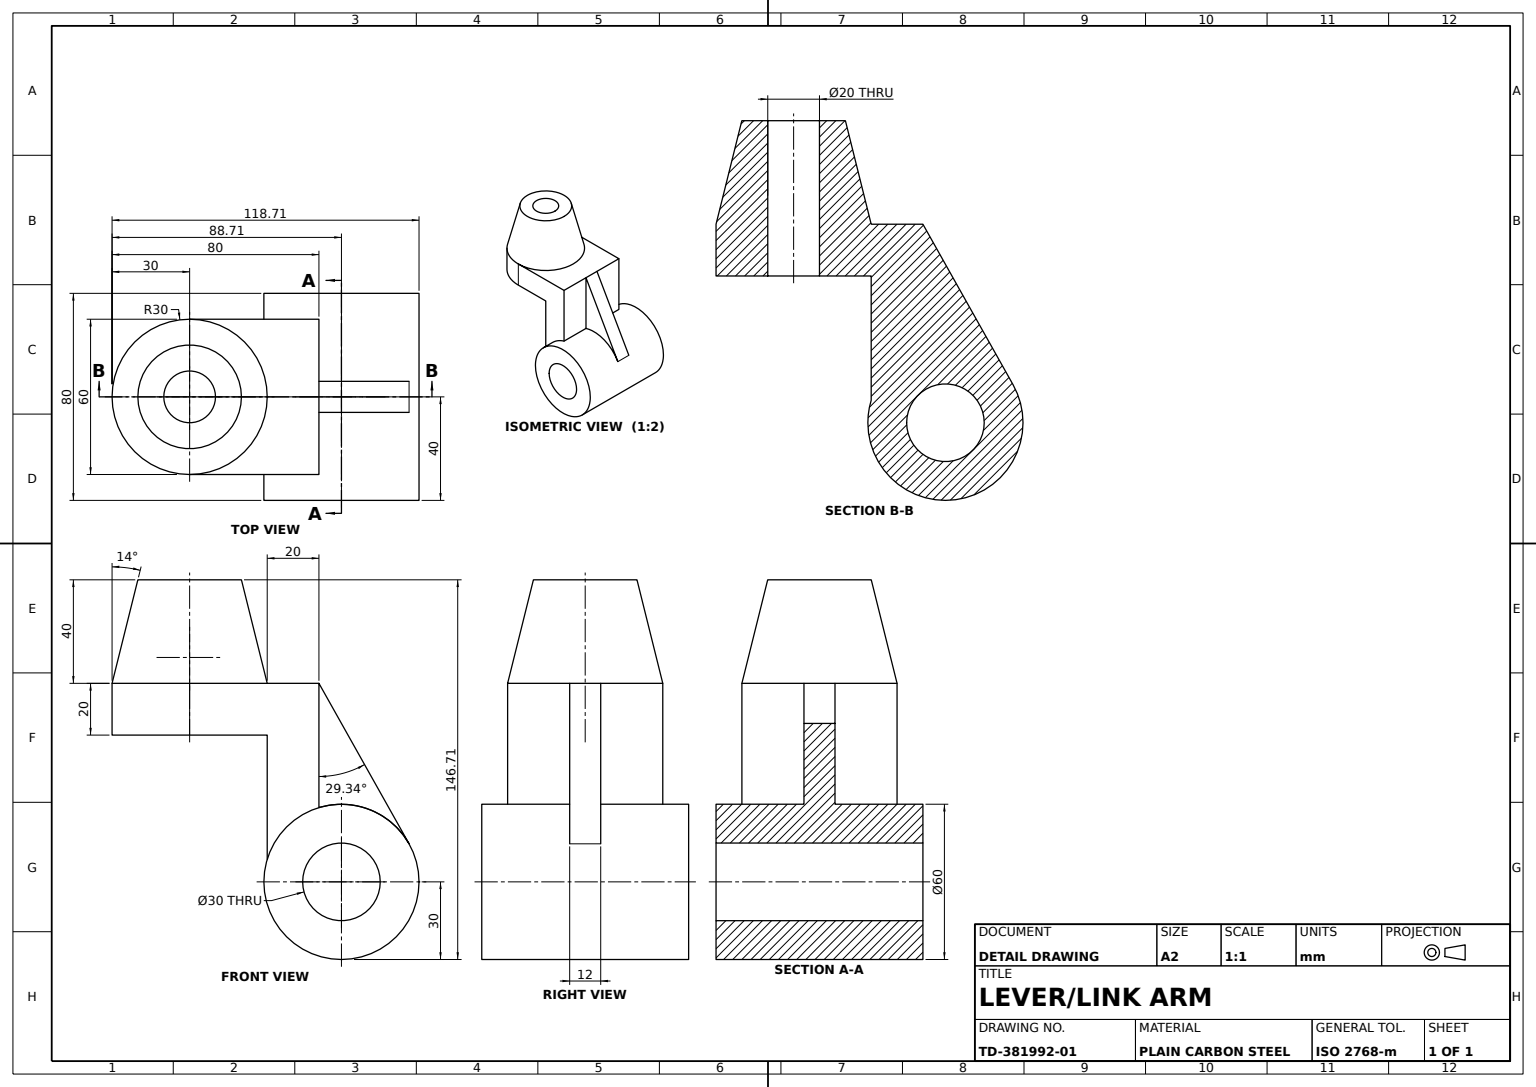
SolidWorks part; units mm, degrees
material "Plain Carbon Steel"
ref_plane "Front Plane" through (0, 0, 0) normal (0, 0, 1) x (1, 0, 0)
ref_plane "Top Plane" through (0, 0, 0) normal (0, 1, 0) x (1, 0, 0)
ref_plane "Right Plane" through (0, 0, 0) normal (1, 0, 0) x (0, 0, -1)
sketch "Base Block Sketch" plane through (0, 0, 0) normal (0, 0, 1) x (1, 0, 0)
  line L0 (0, 94.6468) -> (0, -119.5047) construction
  line L1 (205.6236, 0) -> (-234.7764, 0) construction
  circle A0 centre (0, 0) radius 30
  circle A1 centre (0, 0) radius 15
  dimension "D1" = 60
  dimension "D2" = 30
extrude "Base Block" add sketch "Base Block Sketch" along normal mid plane 80
sketch "Arm Profile Sketch" plane through (0, 0, 0) normal (0, 0, 1) x (1, 0, 0)
  line L0 (-28.7083, 8.7083) -> (-28.7083, 56.7083)
  line L1 (-28.7083, 56.7083) -> (-88.7083, 56.7083)
  line L2 (-88.7083, 56.7083) -> (-88.7083, 76.7083)
  line L3 (-88.7083, 76.7083) -> (-8.7083, 76.7083)
  line L4 (-8.7083, 76.7083) -> (-8.7083, 28.7083)
  circle A1 centre (0, 0) radius 30 construction
  arc A3 (-8.7083, 28.7083) -> (-28.7083, 8.7083) centre (0, 0) ccw
  dimension "D1" = 48
  dimension "D2" = 20
  dimension "D3" = 80
  dimension "D4" = 60
  dimension "D5" = 48
extrude "Arm" add sketch "Arm Profile Sketch" along normal mid plane 60
sketch "Support Rib Sketch" plane through (0, 0, 0) normal (0, 0, 1) x (1, 0, 0)
  line L0 (-8.7083, 76.7083) -> (26.1508, 14.7015)
  line L1 (-8.7083, 76.7083) -> (-8.7083, 28.7083)
  circle A0 centre (0, 0) radius 30 construction
  arc A1 (26.1508, 14.7015) -> (-8.7083, 28.7083) centre (0, 0) ccw
extrude "Support Rib" add sketch "Support Rib Sketch" along normal mid plane 12 contours L0 A1 L1
sketch "Profile Cut Sketch" plane through (0, 76.7083, 0) normal (0, 1, 0) x (1, 0, 0)
  line L0 (-88.7083, -30) -> (-88.7083, 30) construction
  line L4 (-58.7083, 30) -> (-58.7083, -30)
  line L5 (-8.7083, 30) -> (-88.7083, 30) construction
  line L6 (-8.7083, -30) -> (-88.7083, -30) construction
  line L7 (-58.7083, -30) -> (-88.7083, -30)
  line L8 (-88.7083, -30) -> (-88.7083, 30)
  line L9 (-88.7083, 30) -> (-58.7083, 30)
  arc A0 (-58.7083, 30) -> (-58.7083, -30) centre (-58.7083, 0) ccw
  line M4 (-8.7083, 30) -> (-88.7083, 30)
  line M5 (-88.7083, 30) -> (-88.7083, -30)
  line M6 (-88.7083, -30) -> (-8.7083, -30)
  dimension "D1" = 30
extrude "Profile Cut" cut sketch "Profile Cut Sketch" against normal through all contours A0 L8 M6 | A0 M4 M5
sketch "Drafted Boss Sketch" plane through (0, 76.7083, 0) normal (0, 1, 0) x (1, 0, 0)
  circle A0 centre (-58.7083, 0) radius 30
extrude "Drafted Cylindrical Boss" add sketch "Drafted Boss Sketch" along normal blind 40 draft 14
sketch "Boss Bore Sketch" plane through (0, 116.7083, 0) normal (0, 1, 0) x (1, 0, 0)
  circle A0 centre (-58.7083, 0) radius 10
  dimension "D1" = 20
extrude "Boss Bore Ø20" cut sketch "Boss Bore Sketch" against normal through all
